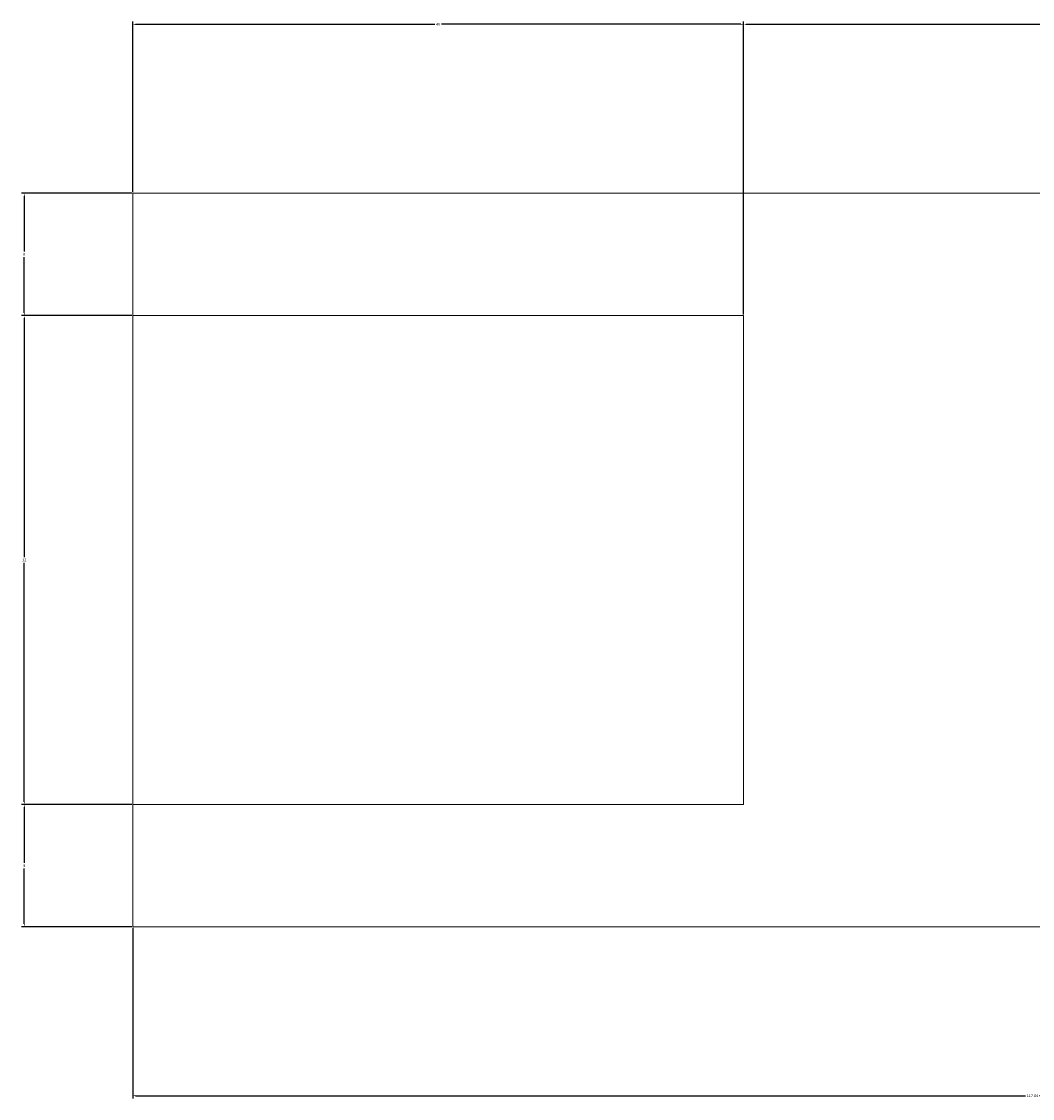
# Model space of a CAD drawing. Units: millimetres. Extents: x 4402 to 4534, y 1655 to 1725.
# Tile 1 of 2: x 4402 to 4468, y 1655 to 1725. Entities that reach past the tile are written whole.
import ezdxf

# ---------------------------------------------------------------- set-up
doc = ezdxf.new("R2010")
doc.units = ezdxf.units.MM
doc.layers.add('M-CONS', color=8, linetype='Continuous', lineweight=18)
doc.layers.add('M-DIMS', color=2, linetype='Continuous', lineweight=18)
doc.styles.get("Standard").update_dxf_attribs({"font": 'arial.ttf'})
doc.dimstyles.get("Standard").update_dxf_attribs({"dimtxt": 0.18, "dimasz": 0.18, "dimexe": 0.18, "dimexo": 0.0625, "dimgap": 0.09, "dimtad": 0, "dimtih": 1, "dimtoh": 1, "dimdec": 4, "dimzin": 0, "dimdsep": 46, "dimtxsty": 'Standard', "dimcen": 0.09, "dimadec": 0, "dimazin": 0, "dimtfac": 1, "dimtdec": 4, "dimtofl": 0, "dimtmove": 0, "dimatfit": 3, "dimfxl": 1, "dimtolj": 1, "dimtzin": 0, "dimarcsym": 0})

# ---------------------------------------------------------------- blocks, each defined once
blk = doc.blocks.new('*D1')
at = {"layer": 'Defpoints', "color": 0, "transparency": 16777216}
for p in [(4401.738, 1705.994), (4408.838, 1705.994), (4408.838, 1673.994)]:
    blk.add_point(p, dxfattribs=at)
at = {"layer": 'M-DIMS', "color": 0, "lineweight": -2, "transparency": 16777216}
for p, q in [((4408.775, 1705.994), (4401.558, 1705.994)), ((4401.738, 1705.814), (4401.738, 1690.176)), ((4401.738, 1674.174), (4401.738, 1689.812)), ((4408.775, 1673.994), (4401.558, 1673.994))]:
    blk.add_line(p, q, dxfattribs=at)
at = {"layer": 'M-DIMS', "color": 0, "transparency": 16777216}
for points in [[(4401.708, 1705.814), (4401.768, 1705.814), (4401.738, 1705.994)], [(4401.708, 1674.174), (4401.768, 1674.174), (4401.738, 1673.994)]]:
    blk.add_solid(points, dxfattribs=at)
at = {"layer": 'M-DIMS', "color": 0, "transparency": 16777216, "insert": (4401.738, 1689.994), "char_height": 0.18, "attachment_point": 5}
blk.add_mtext('\\A1;32', dxfattribs=at)
blk = doc.blocks.new('*D2')
at = {"layer": 'Defpoints', "color": 0, "transparency": 16777216}
for p in [(4401.738, 1673.994), (4408.838, 1673.994), (4408.838, 1665.994)]:
    blk.add_point(p, dxfattribs=at)
at = {"layer": 'M-DIMS', "color": 0, "lineweight": -2, "transparency": 16777216}
for p, q in [((4408.775, 1673.994), (4401.558, 1673.994)), ((4401.738, 1673.814), (4401.738, 1670.176)), ((4401.738, 1666.174), (4401.738, 1669.812)), ((4408.775, 1665.994), (4401.558, 1665.994))]:
    blk.add_line(p, q, dxfattribs=at)
at = {"layer": 'M-DIMS', "color": 0, "transparency": 16777216}
for points in [[(4401.708, 1673.814), (4401.768, 1673.814), (4401.738, 1673.994)], [(4401.708, 1666.174), (4401.768, 1666.174), (4401.738, 1665.994)]]:
    blk.add_solid(points, dxfattribs=at)
at = {"layer": 'M-DIMS', "color": 0, "transparency": 16777216, "insert": (4401.738, 1669.994), "char_height": 0.18, "attachment_point": 5}
blk.add_mtext('\\A1;8', dxfattribs=at)
blk = doc.blocks.new('*D3')
at = {"layer": 'Defpoints', "color": 0, "transparency": 16777216}
for p in [(4401.738, 1713.994), (4408.838, 1713.994), (4408.838, 1705.994)]:
    blk.add_point(p, dxfattribs=at)
at = {"layer": 'M-DIMS', "color": 0, "lineweight": -2, "transparency": 16777216}
for p, q in [((4408.775, 1713.994), (4401.558, 1713.994)), ((4401.738, 1713.814), (4401.738, 1710.176)), ((4401.738, 1706.174), (4401.738, 1709.812)), ((4408.775, 1705.994), (4401.558, 1705.994))]:
    blk.add_line(p, q, dxfattribs=at)
at = {"layer": 'M-DIMS', "color": 0, "transparency": 16777216}
for points in [[(4401.708, 1713.814), (4401.768, 1713.814), (4401.738, 1713.994)], [(4401.708, 1706.174), (4401.768, 1706.174), (4401.738, 1705.994)]]:
    blk.add_solid(points, dxfattribs=at)
at = {"layer": 'M-DIMS', "color": 0, "transparency": 16777216, "insert": (4401.738, 1709.994), "char_height": 0.18, "attachment_point": 5}
blk.add_mtext('\\A1;8', dxfattribs=at)
blk = doc.blocks.new('*D4')
at = {"layer": 'Defpoints', "color": 0, "transparency": 16777216}
for p in [(4448.838, 1725.054), (4408.838, 1713.994), (4448.838, 1705.994)]:
    blk.add_point(p, dxfattribs=at)
at = {"layer": 'M-DIMS', "color": 0, "lineweight": -2, "transparency": 16777216}
for p, q in [((4408.838, 1714.057), (4408.838, 1725.234)), ((4409.018, 1725.054), (4428.616, 1725.054)), ((4448.658, 1725.054), (4429.06, 1725.054)), ((4448.838, 1706.057), (4448.838, 1725.234))]:
    blk.add_line(p, q, dxfattribs=at)
at = {"layer": 'M-DIMS', "color": 0, "transparency": 16777216}
for points in [[(4409.018, 1725.084), (4409.018, 1725.024), (4408.838, 1725.054)], [(4448.658, 1725.084), (4448.658, 1725.024), (4448.838, 1725.054)]]:
    blk.add_solid(points, dxfattribs=at)
at = {"layer": 'M-DIMS', "color": 0, "transparency": 16777216, "insert": (4428.838, 1725.054), "char_height": 0.18, "attachment_point": 5}
blk.add_mtext('\\A1;40', dxfattribs=at)
blk = doc.blocks.new('*D5')
at = {"layer": 'Defpoints', "color": 0, "transparency": 16777216}
for p in [(4526.677, 1686.994), (4408.838, 1665.994), (4526.677, 1654.934)]:
    blk.add_point(p, dxfattribs=at)
at = {"layer": 'M-DIMS', "color": 0, "lineweight": -2, "transparency": 16777216}
for p, q in [((4526.677, 1686.932), (4526.677, 1654.754)), ((4408.838, 1665.932), (4408.838, 1654.754)), ((4409.018, 1654.934), (4467.303, 1654.934)), ((4526.497, 1654.934), (4468.212, 1654.934))]:
    blk.add_line(p, q, dxfattribs=at)
at = {"layer": 'M-DIMS', "color": 0, "transparency": 16777216}
for points in [[(4409.018, 1654.964), (4409.018, 1654.904), (4408.838, 1654.934)], [(4526.497, 1654.964), (4526.497, 1654.904), (4526.677, 1654.934)]]:
    blk.add_solid(points, dxfattribs=at)
at = {"layer": 'M-DIMS', "color": 0, "transparency": 16777216, "insert": (4467.757, 1654.934), "char_height": 0.18, "attachment_point": 5}
blk.add_mtext('\\A1;117.84', dxfattribs=at)
blk = doc.blocks.new('*D6')
at = {"layer": 'Defpoints', "color": 0, "transparency": 16777216}
for p in [(4498.838, 1725.054), (4448.838, 1705.994), (4498.838, 1689.994)]:
    blk.add_point(p, dxfattribs=at)
at = {"layer": 'M-DIMS', "color": 0, "lineweight": -2, "transparency": 16777216}
for p, q in [((4448.838, 1706.057), (4448.838, 1725.234)), ((4449.018, 1725.054), (4473.619, 1725.054)), ((4498.658, 1725.054), (4474.057, 1725.054)), ((4498.838, 1690.057), (4498.838, 1725.234))]:
    blk.add_line(p, q, dxfattribs=at)
at = {"layer": 'M-DIMS', "color": 0, "transparency": 16777216}
for points in [[(4449.018, 1725.084), (4449.018, 1725.024), (4448.838, 1725.054)], [(4498.658, 1725.084), (4498.658, 1725.024), (4498.838, 1725.054)]]:
    blk.add_solid(points, dxfattribs=at)
at = {"layer": 'M-DIMS', "color": 0, "transparency": 16777216, "insert": (4473.838, 1725.054), "char_height": 0.18, "attachment_point": 5}
blk.add_mtext('\\A1;50', dxfattribs=at)

msp = doc.modelspace()

# ---------------------------------------------------------------- linework, layer by layer
at = {"layer": 'M-CONS'}
msp.add_line((4408.838, 1689.994), (4408.838, 1689.994), dxfattribs=at)
for points in [[(4484.416, 1665.994), (4408.838, 1665.994), (4408.838, 1713.994), (4484.416, 1713.994)], [(4408.838, 1705.994), (4448.838, 1705.994), (4448.838, 1673.994), (4408.838, 1673.994)]]:
    msp.add_lwpolyline(points, dxfattribs=at)

# ---------------------------------------------------------------- dimensions: what is measured, and where the dimension line sits
at = {"layer": 'M-DIMS'}
for base, p1, p2, override, picture, middle in [((4448.838, 1725.054), (4408.838, 1713.994), (4448.838, 1705.994), {"dimdec": 0, "dimlfac": 1, "dimrnd": 0, "dimzin": 0, "dimdsep": 46, "dimlunit": 2}, '*D4', (4428.838, 1725.054)), ((4498.838, 1725.054), (4448.838, 1705.994), (4498.838, 1689.994), {"dimdec": 0, "dimlfac": 1, "dimrnd": 0, "dimzin": 0, "dimdsep": 46, "dimlunit": 2}, '*D6', (4473.838, 1725.054)), ((4526.677, 1654.934), (4408.838, 1665.994), (4526.677, 1686.994), {"dimdec": 2, "dimlfac": 1, "dimrnd": 0, "dimzin": 0, "dimdsep": 46, "dimlunit": 2}, '*D5', (4467.757, 1654.934))]:
    dim = msp.add_linear_dim(base=base, p1=p1, p2=p2, dimstyle='Standard', override=override, dxfattribs=at)
    dim.commit()
    dim.dimension.update_dxf_attribs({"geometry": picture, "text_midpoint": middle})
for base, p1, p2, picture, middle in [((4401.738, 1713.994), (4408.838, 1705.994), (4408.838, 1713.994), '*D3', (4401.738, 1709.994)), ((4401.738, 1705.994), (4408.838, 1673.994), (4408.838, 1705.994), '*D1', (4401.738, 1689.994)), ((4401.738, 1673.994), (4408.838, 1665.994), (4408.838, 1673.994), '*D2', (4401.738, 1669.994))]:
    dim = msp.add_linear_dim(base=base, p1=p1, p2=p2, angle=90, dimstyle='Standard', override={"dimdec": 0, "dimlfac": 1, "dimrnd": 0, "dimzin": 0, "dimdsep": 46, "dimlunit": 2}, dxfattribs=at)
    dim.commit()
    dim.dimension.update_dxf_attribs({"geometry": picture, "text_midpoint": middle})

doc.saveas('drawing.dxf')
